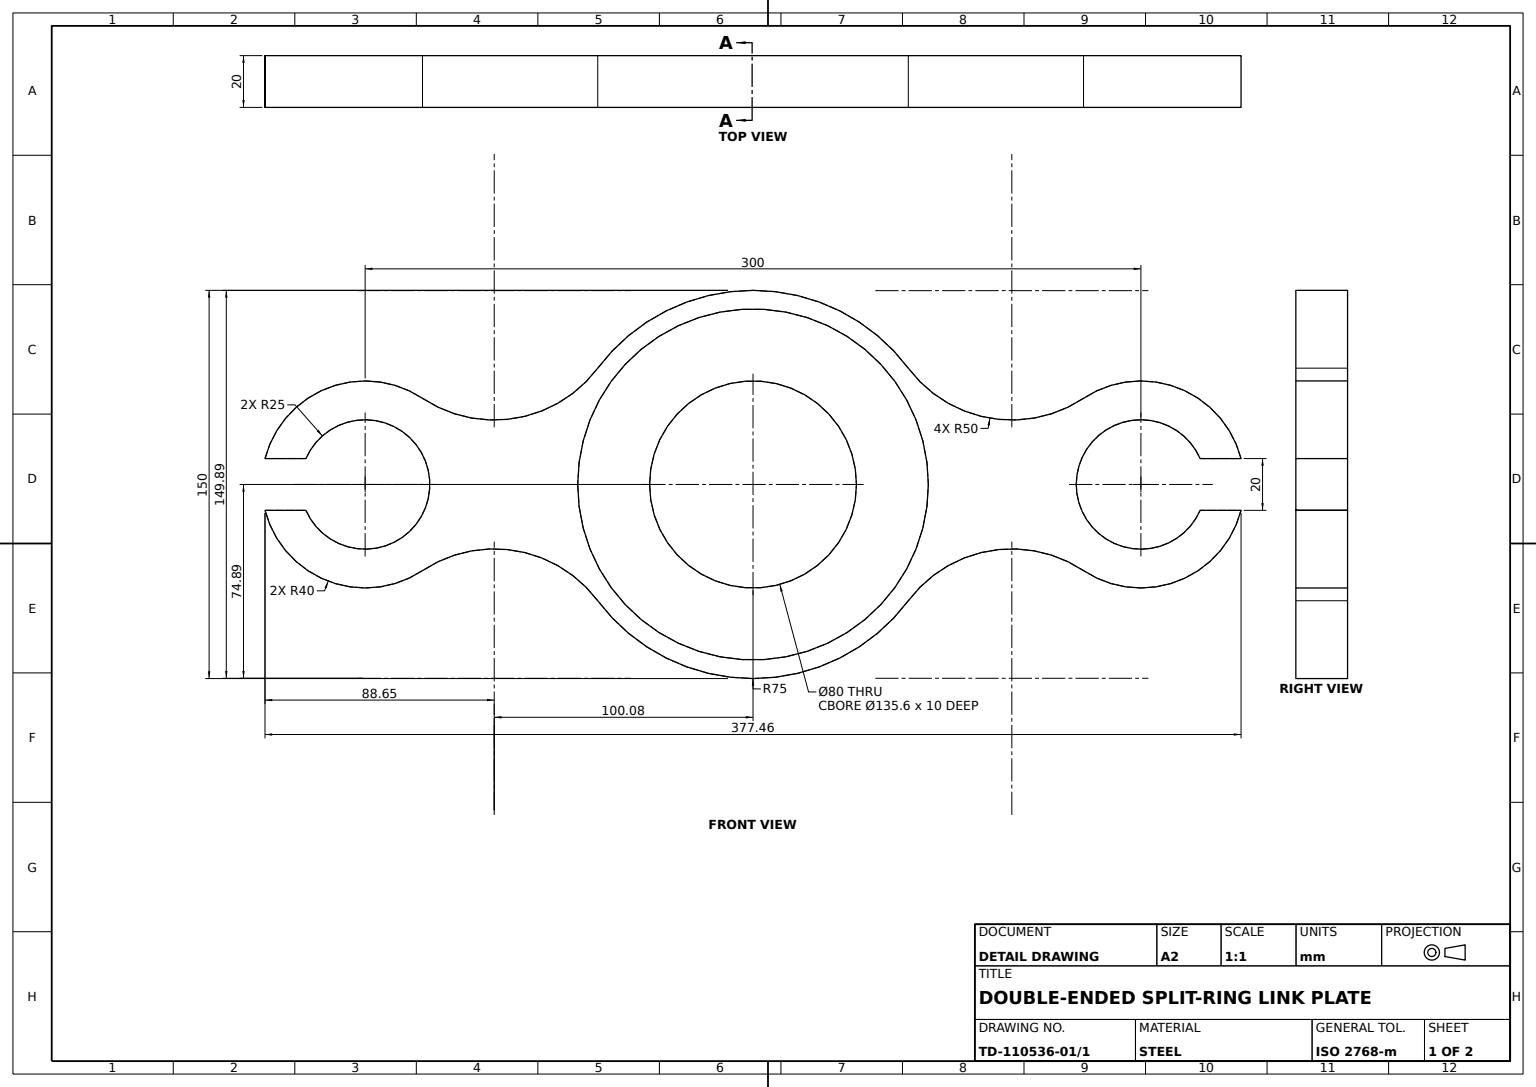
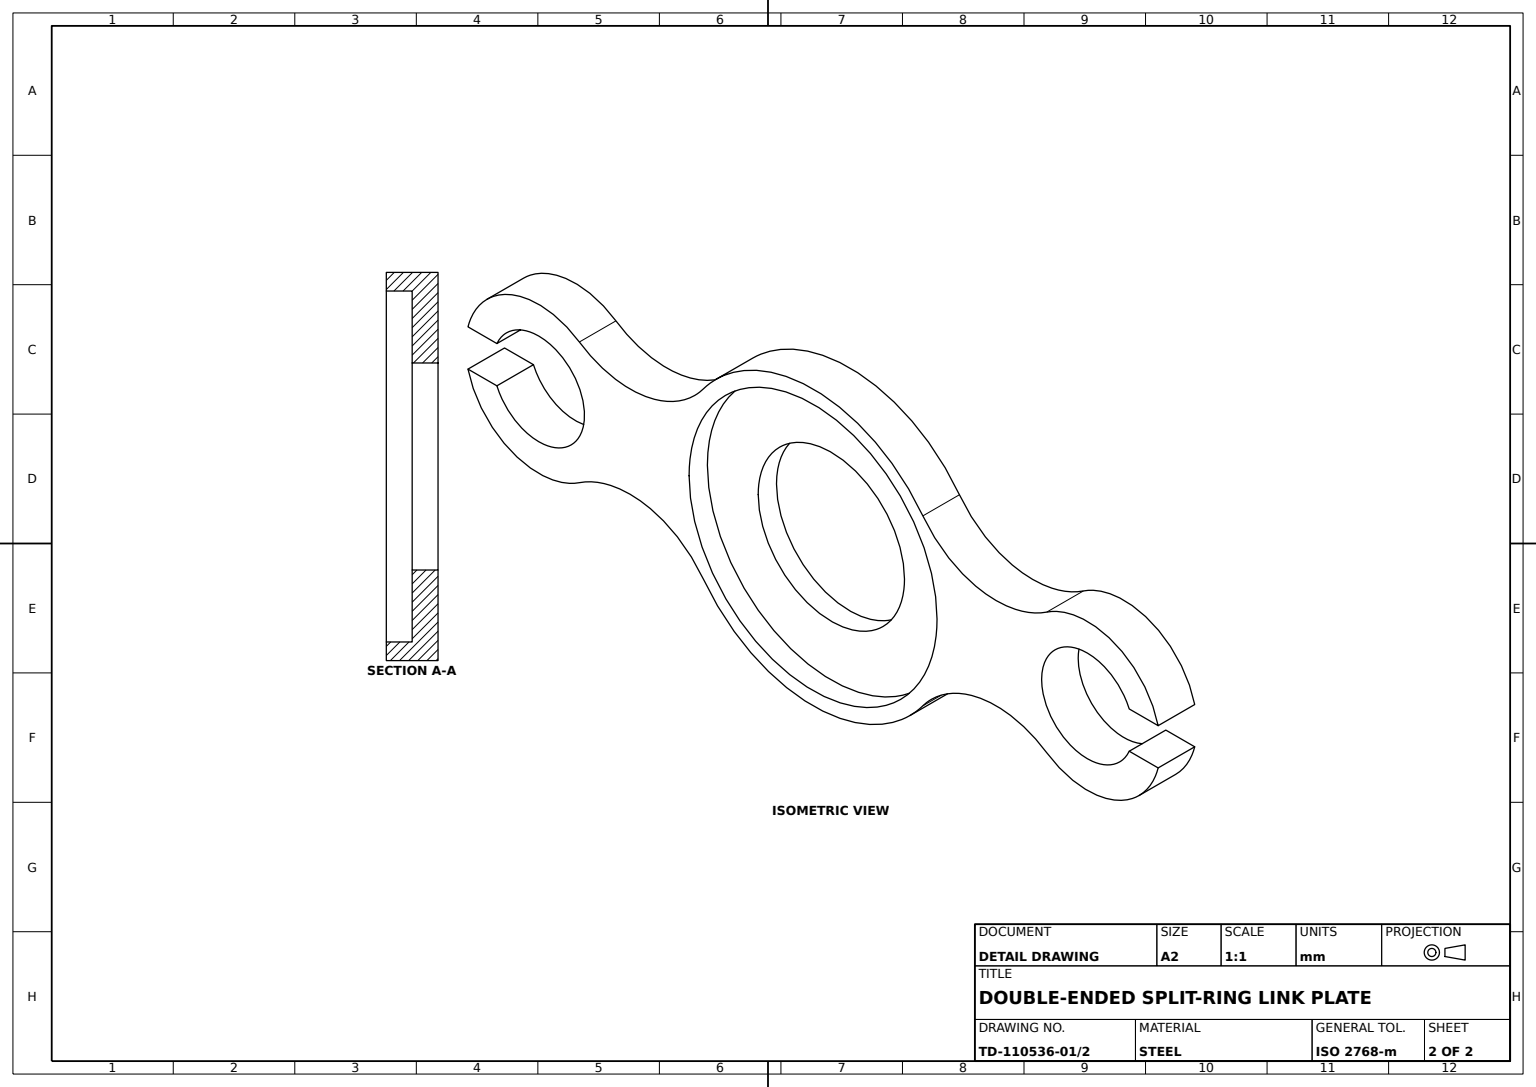
SolidWorks part; units mm, degrees
material "Plain Carbon Steel"
ref_plane "Front Plane" through (0, 0, 0) normal (0, 0, 1) x (1, 0, 0)
ref_plane "Top Plane" through (0, 0, 0) normal (0, 1, 0) x (1, 0, 0)
ref_plane "Right Plane" through (0, 0, 0) normal (1, 0, 0) x (0, 0, -1)
sketch "Link Plate Outline Sketch" plane through (0, 0, 0) normal (0, 0, 1) x (1, 0, 0)
  line L0 (0, 0) -> (150, 0) construction
  line L1 (150, 0) -> (300, 0) construction
  line L2 (0, 0) -> (-40, 0) construction
  line L3 (300, 0) -> (367.9585, 0) construction
  line L4 (-38.7298, 10) -> (-22.9129, 10) construction
  line L5 (-38.7298, 10) -> (-22.9129, 10)
  line L7 (-38.7298, -10) -> (-22.9129, -10)
  line L8 (338.7298, 10) -> (322.9129, 10)
  line L11 (322.9129, -10) -> (338.7298, -10)
  arc A0 (-22.9129, -10) -> (-22.9129, 10) centre (0, 0) ccw
  arc A1 (-38.7298, -10) -> (22.1852, -33.2839) centre (0, 0) ccw
  arc A3 (322.9129, 10) -> (322.9129, -10) centre (300, 0) ccw
  arc A6 (338.7298, 10) -> (277.8148, 33.2839) centre (300, 0) ccw
  arc A7 (210.05, 44.9333) -> (89.95, 44.9333) centre (150, 0) ccw
  arc A8 (22.1852, 33.2839) -> (89.95, 44.9333) centre (49.9167, 74.8888) ccw
  arc A9 (22.1852, -33.2839) -> (89.95, -44.9333) centre (49.9167, -74.8888) cw
  arc A10 (210.05, 44.9333) -> (277.8148, 33.2839) centre (250.0833, 74.8888) ccw
  arc A11 (210.05, -44.9333) -> (277.8148, -33.2839) centre (250.0833, -74.8888) cw
  arc A12 (89.95, -44.9333) -> (210.05, -44.9333) centre (150, 0) ccw
  arc A13 (22.1852, 33.2839) -> (-38.7298, 10) centre (0, 0) ccw
  arc A14 (277.8148, -33.2839) -> (338.7298, -10) centre (300, 0) ccw
  dimension "D1" = 50
  dimension "D2" = 80
  dimension "D4" = 80
  dimension "D5" = 50
  dimension "D6" = 150
  dimension "D10" = 50
  dimension "D11" = 50
  dimension "D12" = 50
  dimension "D13" = 50
  dimension "D3" = 150
  dimension "D7" = 300
  dimension "D8" = 15.817
  dimension "D9" = 15.817
  dimension "D14" = 15.817
  dimension "D15" = 15.817
extrude "Link Plate 20mm" add sketch "Link Plate Outline Sketch" along normal blind 20
sketch "Centre Opening Sketch" plane through (0, 0, 20) normal (0, 0, 1) x (1, 0, 0)
  circle A0 centre (150, 0) radius 67.8
  dimension "D1" = 135.6
extrude "Centre Opening Ø135.6" cut sketch "Centre Opening Sketch" against normal blind 20
ref_plane "Web Mid Plane" through (0, 0, 10) normal (0, 0, 1) x (1, 0, 0)
sketch "Annular Web Sketch" plane through (0, 0, 10) normal (0, 0, 1) x (1, 0, 0)
  circle A0 centre (150, 0) radius 67.8
  circle A1 centre (150, 0) radius 40
  dimension "D1" = 80
  dimension "D2" = 135.6
extrude "Annular Web Ø80xØ135.6" add sketch "Annular Web Sketch" against normal blind 10
